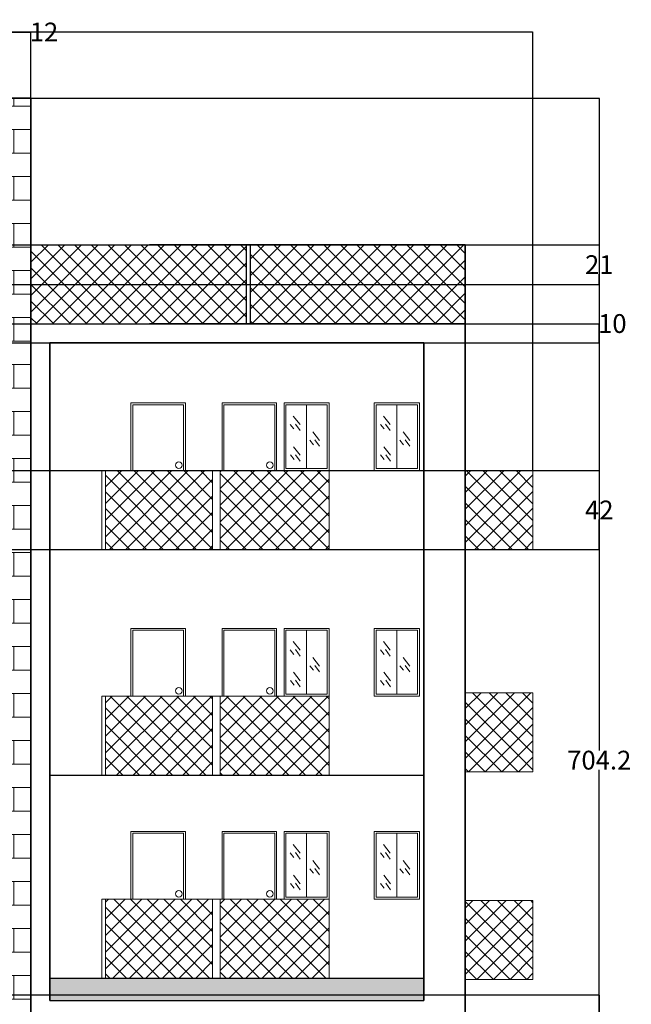
# Model space of a CAD drawing. Units: inches. Extents: x 183 to 891, y 196 to 984.
# Tile 3 of 3: x 566 to 891, y 460 to 984. Entities that reach past the tile are written whole.
import ezdxf

# ---------------------------------------------------------------- set-up
doc = ezdxf.new("R2010")
doc.units = ezdxf.units.IN
doc.header["$MEASUREMENT"] = 0
for name, color, linetype, lineweight in [('A-ANNO-DIMS', 2, 'Continuous', 18), ('A-DOOR', 3, 'Continuous', 20), ('A-FLOR', 7, 'Continuous', 30), ('A-FLOR-PATT', 2, 'Continuous', 13), ('A-GLAZ', 4, 'Continuous', 18), ('A-RAIL', 7, 'Continuous', 20), ('A-RAIL-PATT', 8, 'Continuous', 13), ('A-ROOF', 7, 'Continuous', 25), ('A-WALL', 7, 'Continuous', 35), ('A-WALL-PATT', 251, 'Continuous', 13)]:
    doc.layers.add(name, color=color, linetype=linetype, lineweight=lineweight)
doc.styles.get("Standard").update_dxf_attribs({"font": 'arial.ttf'})
doc.dimstyles.get("Standard").update_dxf_attribs({"dimtxt": 10, "dimasz": 0.18, "dimexe": 0.18, "dimexo": 0.0625, "dimgap": 0.09, "dimtad": 0, "dimtih": 1, "dimtoh": 1, "dimdec": 0, "dimzin": 0, "dimdsep": 46, "dimlunit": 3, "dimtxsty": 'Standard', "dimcen": 0.09, "dimadec": 0, "dimazin": 0, "dimtfac": 1, "dimtdec": 0, "dimtofl": 0, "dimtmove": 0, "dimatfit": 3, "dimfxl": 1, "dimtolj": 1, "dimtzin": 0, "dimarcsym": 0})

# ---------------------------------------------------------------- blocks, each defined once
blk = doc.blocks.new('WIN-SASH-PAIR-22X34')
for p, q in [((11, 34), (11, 0)), ((18.11, 27.96), (14.53, 23.4)), ((16.98, 23.73), (14.53, 20.31)), ((19.74, 23.56), (17.79, 21.12)), ((7.74, 19.54), (4.16, 14.99)), ((6.61, 15.31), (4.16, 11.9)), ((9.37, 15.15), (7.42, 12.71)), ((18.01, 11.64), (14.43, 7.09)), ((16.87, 7.41), (14.43, 4)), ((19.64, 7.25), (17.69, 4.81))]:
    blk.add_line(p, q)
blk.add_lwpolyline([(0, 0), (22, 0), (22, 34), (0, 34)], close=True)
blk = doc.blocks.new('DOOR-BALCONY-ELEV-29')
for p, q in [((0, 0), (0, 36)), ((0, 36), (29, 36)), ((1, 35), (28, 35)), ((1, 0), (1, 35)), ((28, 35), (28, 0)), ((29, 36), (29, 0))]:
    blk.add_line(p, q)
blk.add_circle((3.53, 2.84), 1.74)
blk = doc.blocks.new('*D8')
at = {"layer": 'A-ANNO-DIMS', "color": 0, "lineweight": -2, "transparency": 16777216}
for p, q in [((238.6, 742.93), (238.6, 977.12)), ((238.78, 976.94), (527.45, 976.94)), ((838.42, 976.94), (549.75, 976.94)), ((838.6, 743.74), (838.6, 977.12))]:
    blk.add_line(p, q, dxfattribs=at)
at = {"layer": 'A-ANNO-DIMS', "color": 0, "transparency": 16777216}
for points in [[(238.78, 976.97), (238.78, 976.91), (238.6, 976.94)], [(838.42, 976.97), (838.42, 976.91), (838.6, 976.94)]]:
    blk.add_solid(points, dxfattribs=at)
at = {"layer": 'Defpoints', "color": 0, "transparency": 16777216}
for p in [(838.6, 976.94), (238.6, 742.86), (838.6, 743.68)]:
    blk.add_point(p, dxfattribs=at)
at = {"layer": 'A-ANNO-DIMS', "color": 0, "transparency": 16777216, "insert": (538.6, 976.94), "char_height": 10, "attachment_point": 5}
blk.add_mtext('\\A1;600', dxfattribs=at)
blk = doc.blocks.new('*D9')
at = {"layer": 'A-ANNO-DIMS', "color": 0, "lineweight": -2, "transparency": 16777216}
for p, q in [((571.66, 941.68), (874.04, 941.68)), ((873.86, 941.5), (873.86, 594.79)), ((873.86, 237.69), (873.86, 584.4)), ((802.66, 237.51), (874.04, 237.51))]:
    blk.add_line(p, q, dxfattribs=at)
at = {"layer": 'A-ANNO-DIMS', "color": 0, "transparency": 16777216}
for points in [[(873.83, 941.5), (873.89, 941.5), (873.86, 941.68)], [(873.83, 237.69), (873.89, 237.69), (873.86, 237.51)]]:
    blk.add_solid(points, dxfattribs=at)
at = {"layer": 'Defpoints', "color": 0, "transparency": 16777216}
for p in [(571.6, 941.68), (873.86, 941.68), (802.6, 237.51)]:
    blk.add_point(p, dxfattribs=at)
at = {"layer": 'A-ANNO-DIMS', "color": 0, "transparency": 16777216, "insert": (873.86, 589.59), "char_height": 10, "attachment_point": 5}
blk.add_mtext('\\A1;704.2', dxfattribs=at)
blk = doc.blocks.new('*D37')
at = {"layer": 'A-ANNO-DIMS', "color": 0, "lineweight": -2, "transparency": 16777216}
for p, q in [((559.6, 317.74), (559.6, 977.12)), ((559.78, 976.94), (571.42, 976.94)), ((571.6, 237.57), (571.6, 977.12)), ((571.6, 976.94), (571.78, 976.94))]:
    blk.add_line(p, q, dxfattribs=at)
at = {"layer": 'A-ANNO-DIMS', "color": 0, "transparency": 16777216}
for points in [[(559.78, 976.97), (559.78, 976.91), (559.6, 976.94)], [(571.42, 976.97), (571.42, 976.91), (571.6, 976.94)]]:
    blk.add_solid(points, dxfattribs=at)
at = {"layer": 'Defpoints', "color": 0, "transparency": 16777216}
for p in [(571.6, 976.94), (559.6, 317.68), (571.6, 237.51)]:
    blk.add_point(p, dxfattribs=at)
at = {"layer": 'A-ANNO-DIMS', "color": 0, "transparency": 16777216, "insert": (578.51, 976.94), "char_height": 10, "attachment_point": 5}
blk.add_mtext('\\A1;12', dxfattribs=at)
blk = doc.blocks.new('*D39')
at = {"layer": 'A-ANNO-DIMS', "color": 0, "lineweight": -2, "transparency": 16777216}
for p, q in [((559.66, 464.68), (874.04, 464.68)), ((873.86, 464.5), (873.86, 396.29)), ((873.86, 317.86), (873.86, 386.06)), ((559.66, 317.68), (874.04, 317.68))]:
    blk.add_line(p, q, dxfattribs=at)
at = {"layer": 'A-ANNO-DIMS', "color": 0, "transparency": 16777216}
for points in [[(873.83, 464.5), (873.89, 464.5), (873.86, 464.68)], [(873.83, 317.86), (873.89, 317.86), (873.86, 317.68)]]:
    blk.add_solid(points, dxfattribs=at)
at = {"layer": 'Defpoints', "color": 0, "transparency": 16777216}
for p in [(559.6, 464.68), (873.86, 464.68), (559.6, 317.68)]:
    blk.add_point(p, dxfattribs=at)
at = {"layer": 'A-ANNO-DIMS', "color": 0, "transparency": 16777216, "insert": (873.86, 391.18), "char_height": 10, "attachment_point": 5}
blk.add_mtext('\\A1;147', dxfattribs=at)
blk = doc.blocks.new('*D45')
at = {"layer": 'A-ANNO-DIMS', "color": 0, "lineweight": -2, "transparency": 16777216}
for p, q in [((467.66, 743.68), (874.04, 743.68)), ((873.86, 743.5), (873.86, 727.79)), ((873.86, 701.86), (873.86, 717.56)), ((467.66, 701.68), (874.04, 701.68))]:
    blk.add_line(p, q, dxfattribs=at)
at = {"layer": 'A-ANNO-DIMS', "color": 0, "transparency": 16777216}
for points in [[(873.83, 743.5), (873.89, 743.5), (873.86, 743.68)], [(873.83, 701.86), (873.89, 701.86), (873.86, 701.68)]]:
    blk.add_solid(points, dxfattribs=at)
at = {"layer": 'Defpoints', "color": 0, "transparency": 16777216}
for p in [(467.6, 743.68), (873.86, 743.68), (467.6, 701.68)]:
    blk.add_point(p, dxfattribs=at)
at = {"layer": 'A-ANNO-DIMS', "color": 0, "transparency": 16777216, "insert": (873.86, 722.68), "char_height": 10, "attachment_point": 5}
blk.add_mtext('\\A1;42', dxfattribs=at)
blk = doc.blocks.new('*D48')
at = {"layer": 'A-ANNO-DIMS', "color": 0, "lineweight": -2, "transparency": 16777216}
for p, q in [((499.66, 821.68), (874.04, 821.68)), ((873.86, 821.68), (873.86, 821.86)), ((873.86, 821.86), (874.04, 821.86)), ((873.86, 811.86), (873.86, 821.5)), ((489.66, 811.68), (874.04, 811.68))]:
    blk.add_line(p, q, dxfattribs=at)
at = {"layer": 'A-ANNO-DIMS', "color": 0, "transparency": 16777216}
for points in [[(873.83, 821.5), (873.89, 821.5), (873.86, 821.68)], [(873.83, 811.86), (873.89, 811.86), (873.86, 811.68)]]:
    blk.add_solid(points, dxfattribs=at)
at = {"layer": 'Defpoints', "color": 0, "transparency": 16777216}
for p in [(499.6, 821.68), (873.86, 821.68), (489.6, 811.68)]:
    blk.add_point(p, dxfattribs=at)
at = {"layer": 'A-ANNO-DIMS', "color": 0, "transparency": 16777216, "insert": (880.81, 821.86), "char_height": 10, "attachment_point": 5}
blk.add_mtext('\\A1;10', dxfattribs=at)
blk = doc.blocks.new('*D49')
at = {"layer": 'A-ANNO-DIMS', "color": 0, "lineweight": -2, "transparency": 16777216}
for p, q in [((499.66, 863.68), (874.04, 863.68)), ((873.86, 863.5), (873.86, 858.29)), ((873.86, 842.86), (873.86, 848.06)), ((499.66, 842.68), (874.04, 842.68))]:
    blk.add_line(p, q, dxfattribs=at)
at = {"layer": 'A-ANNO-DIMS', "color": 0, "transparency": 16777216}
for points in [[(873.83, 863.5), (873.89, 863.5), (873.86, 863.68)], [(873.83, 842.86), (873.89, 842.86), (873.86, 842.68)]]:
    blk.add_solid(points, dxfattribs=at)
at = {"layer": 'Defpoints', "color": 0, "transparency": 16777216}
for p in [(499.6, 863.68), (873.86, 863.68), (499.6, 842.68)]:
    blk.add_point(p, dxfattribs=at)
at = {"layer": 'A-ANNO-DIMS', "color": 0, "transparency": 16777216, "insert": (873.86, 853.18), "char_height": 10, "attachment_point": 5}
blk.add_mtext('\\A1;21', dxfattribs=at)

msp = doc.modelspace()

# ---------------------------------------------------------------- hatches: boundary and pattern name
at = {"layer": 'A-FLOR-PATT'}
h = msp.add_hatch(color=256, dxfattribs=at)
h.dxf.hatch_style = 1
h.paths.add_polyline_path([(489.599, 473.6754), (296.599, 473.6754), (296.599, 461.6754), (489.599, 461.6754)])
h.paths.add_polyline_path([(780.599, 473.6754), (581.599, 473.6754), (581.599, 461.6754), (780.599, 461.6754)])
at = {"layer": 'A-RAIL-PATT'}
h = msp.add_hatch(dxfattribs=at)
h.set_pattern_fill('ANSI37', color=256, scale=50)
h.paths.add_polyline_path([(386.099, 842.6754), (274.599, 842.6754), (274.599, 821.6754), (386.099, 821.6754)])
h.paths.add_polyline_path([(386.099, 863.6754), (274.599, 863.6754), (274.599, 842.6754), (386.099, 842.6754)])
h.paths.add_polyline_path([(499.599, 863.6754), (388.099, 863.6754), (388.099, 842.6754), (499.599, 842.6754)])
h.paths.add_polyline_path([(499.599, 842.6754), (388.099, 842.6754), (388.099, 821.6754), (499.599, 821.6754)])
h.paths.add_polyline_path([(686.099, 863.6754), (571.599, 863.6754), (571.599, 842.6754), (686.099, 842.6754)])
h.paths.add_polyline_path([(686.099, 842.6754), (571.599, 842.6754), (571.599, 821.6754), (634.599, 821.6754), (686.099, 821.6754)])
h.paths.add_polyline_path([(802.599, 863.6754), (688.099, 863.6754), (688.099, 842.6754), (802.599, 842.6754)])
h.paths.add_polyline_path([(802.599, 842.6754), (688.099, 842.6754), (688.099, 821.6754), (802.599, 821.6754)])
h = msp.add_hatch(dxfattribs=at)
h.set_pattern_fill('ANSI37', color=256, scale=50)
h.paths.add_polyline_path([(404.599, 743.6754), (346.599, 743.6754), (346.599, 701.6754), (404.599, 701.6754)])
h.paths.add_polyline_path([(465.599, 743.6754), (408.599, 743.6754), (408.599, 701.6754), (465.599, 701.6754)])
h.paths.add_polyline_path([(668.2227, 743.6754), (611.2227, 743.6754), (611.2227, 701.6754), (668.2227, 701.6754)])
h.paths.add_polyline_path([(730.2227, 743.6754), (706.2227, 743.6754), (672.2227, 743.6754), (672.2227, 701.6754), (730.2227, 701.6754)])
h.paths.add_polyline_path([(838.599, 743.6754), (802.599, 743.6754), (802.599, 701.6754), (838.599, 701.6754)])
h.paths.add_polyline_path([(274.599, 742.8641), (238.599, 742.8641), (238.599, 700.8641), (274.599, 700.8641)])
h.paths.add_polyline_path([(274.599, 625.2404), (238.599, 625.2404), (238.599, 583.2404), (274.599, 583.2404)])
h.paths.add_polyline_path([(404.599, 623.6754), (346.599, 623.6754), (346.599, 581.6754), (404.599, 581.6754)])
h.paths.add_polyline_path([(465.599, 623.6754), (408.599, 623.6754), (408.599, 581.6754), (465.599, 581.6754)])
h.paths.add_polyline_path([(668.2227, 623.6754), (611.2227, 623.6754), (611.2227, 581.6754), (668.2227, 581.6754)])
h.paths.add_polyline_path([(730.2227, 623.6754), (672.2227, 623.6754), (672.2227, 581.6754), (730.2227, 581.6754)])
h.paths.add_polyline_path([(838.599, 625.42), (802.599, 625.42), (802.599, 583.42), (838.599, 583.42)])
h.paths.add_polyline_path([(404.599, 515.6754), (346.599, 515.6754), (346.599, 473.6754), (404.599, 473.6754)])
h.paths.add_polyline_path([(465.599, 515.6754), (408.599, 515.6754), (408.599, 473.6754), (465.599, 473.6754)])
h.paths.add_polyline_path([(668.2227, 515.6754), (611.2227, 515.6754), (611.2227, 473.6754), (668.2227, 473.6754)])
h.paths.add_polyline_path([(730.2227, 515.6754), (706.2227, 515.6754), (672.2227, 515.6754), (672.2227, 473.6754), (730.2227, 473.6754)])
h.paths.add_polyline_path([(838.599, 514.8979), (802.599, 514.8979), (802.599, 472.8979), (838.599, 472.8979)])
h.paths.add_polyline_path([(668.2227, 383.6754), (611.2227, 383.6754), (611.2227, 341.6754), (668.2227, 341.6754)])
h.paths.add_polyline_path([(609.2227, 383.6754), (571.599, 383.6754), (571.599, 341.6754), (601.2227, 341.6754), (609.2227, 341.6754)])
h.paths.add_polyline_path([(730.2227, 383.6754), (672.2227, 383.6754), (672.2227, 341.6754), (730.2227, 341.6754)])
h.paths.add_polyline_path([(838.599, 383.6754), (802.599, 383.6754), (802.599, 341.6754), (838.599, 341.6754)])
h.paths.add_polyline_path([(499.599, 383.6754), (467.599, 383.6754), (467.599, 341.6754), (499.599, 341.6754)])
h.paths.add_polyline_path([(465.599, 383.6754), (408.599, 383.6754), (408.599, 341.6754), (465.599, 341.6754)])
h.paths.add_polyline_path([(404.599, 383.6754), (346.599, 383.6754), (346.599, 341.6754), (404.599, 341.6754)])
h.paths.add_polyline_path([(274.599, 383.6754), (238.599, 383.6754), (238.599, 341.6754), (274.599, 341.6754)])
h.paths.add_polyline_path([(274.599, 514.3451), (238.599, 514.3451), (238.599, 472.3451), (274.599, 472.3451)])
at = {"layer": 'A-WALL-PATT'}
h = msp.add_hatch(dxfattribs=at)
h.set_pattern_fill('BRICK', color=256, scale=50)
h.paths.add_polyline_path([(571.599, 341.6754), (571.599, 821.6754), (571.599, 905.6754), (571.599, 941.6754), (499.599, 941.6754), (499.599, 905.6754), (499.599, 821.6754), (499.599, 341.6754), (499.599, 237.5076), (571.599, 237.5076)])
h.paths.add_polyline_path([(511.599, 317.6754), (511.599, 905.6754), (559.599, 905.6754), (559.599, 317.6754)], flags=16)

# ---------------------------------------------------------------- linework, layer by layer
at = {"layer": 'A-FLOR'}
for p, q in [((581.599, 701.6754), (780.599, 701.6754)), ((581.599, 581.6754), (780.599, 581.6754)), ((581.599, 473.6754), (780.599, 473.6754)), ((581.599, 461.6754), (780.599, 461.6754))]:
    msp.add_line(p, q, dxfattribs=at)
at = {"layer": 'A-GLAZ'}
for p, q in [((763.2227, 743.6754), (754.2227, 743.6754)), ((763.2227, 623.6754), (754.2227, 623.6754)), ((763.2227, 515.6754), (754.2227, 515.6754))]:
    msp.add_line(p, q, dxfattribs=at)
for points in [[(730.2227, 743.6754), (706.2227, 743.6754), (706.2227, 779.6754), (730.2227, 779.6754)], [(778.2227, 743.6754), (754.2227, 743.6754), (754.2227, 779.6754), (778.2227, 779.6754)], [(730.2227, 623.6754), (706.2227, 623.6754), (706.2227, 659.6754), (730.2227, 659.6754)], [(778.2227, 623.6754), (754.2227, 623.6754), (754.2227, 659.6754), (778.2227, 659.6754)], [(730.2227, 515.6754), (706.2227, 515.6754), (706.2227, 551.6754), (730.2227, 551.6754)], [(778.2227, 515.6754), (754.2227, 515.6754), (754.2227, 551.6754), (778.2227, 551.6754)]]:
    msp.add_lwpolyline(points, close=True, dxfattribs=at)
at = {"layer": 'A-RAIL'}
for p, q in [((730.2227, 743.6754), (609.2227, 743.6754)), ((609.2227, 701.6754), (609.2227, 743.6754)), ((609.2227, 743.6754), (730.2227, 743.6754)), ((611.2227, 701.6754), (611.2227, 743.6754)), ((668.2227, 743.4954), (668.2227, 701.6754)), ((672.2227, 743.4954), (672.2227, 701.6754)), ((730.2227, 743.6754), (730.2227, 701.6754)), ((838.599, 743.6754), (802.599, 743.6754)), ((838.599, 701.6754), (838.599, 743.6754)), ((802.599, 701.6754), (838.599, 701.6754)), ((609.2227, 623.6754), (730.2227, 623.6754)), ((730.2227, 623.6754), (609.2227, 623.6754)), ((609.2227, 581.6754), (609.2227, 623.6754)), ((611.2227, 581.6754), (611.2227, 623.6754)), ((668.2227, 623.4954), (668.2227, 581.6754)), ((672.2227, 623.4954), (672.2227, 581.6754)), ((730.2227, 623.6754), (730.2227, 581.6754)), ((838.599, 625.42), (802.599, 625.42)), ((838.599, 583.42), (838.599, 625.42)), ((802.599, 583.42), (838.599, 583.42)), ((730.2227, 515.6754), (609.2227, 515.6754)), ((609.2227, 473.6754), (609.2227, 515.6754)), ((611.2227, 473.6754), (611.2227, 515.6754)), ((668.2227, 515.4954), (668.2227, 473.6754)), ((672.2227, 515.4954), (672.2227, 473.6754)), ((730.2227, 515.6754), (730.2227, 473.6754)), ((838.599, 514.8979), (802.599, 514.8979)), ((838.599, 472.8979), (838.599, 514.8979)), ((802.599, 472.8979), (838.599, 472.8979))]:
    msp.add_line(p, q, dxfattribs=at)
at = {"layer": 'A-ROOF'}
for p, q in [((571.599, 863.6754), (634.599, 863.6754)), ((571.599, 863.6754), (802.599, 863.6754)), ((802.599, 863.6754), (634.599, 863.6754)), ((686.099, 863.6754), (686.099, 821.6754)), ((688.099, 863.6754), (688.099, 821.6754)), ((571.599, 842.6754), (802.599, 842.6754)), ((571.599, 821.6754), (634.599, 821.6754)), ((802.599, 821.6754), (634.599, 821.6754))]:
    msp.add_line(p, q, dxfattribs=at)
at = {"layer": 'A-WALL'}
for p, q in [((499.599, 941.6754), (571.599, 941.6754)), ((571.599, 941.6754), (571.599, 905.6754)), ((571.599, 905.6754), (571.599, 821.6754)), ((802.599, 237.5076), (802.599, 863.6754)), ((571.599, 821.6754), (571.599, 341.6754)), ((581.599, 811.6754), (581.599, 461.6754)), ((780.599, 811.6754), (581.599, 811.6754)), ((780.599, 461.6754), (780.599, 811.6754))]:
    msp.add_line(p, q, dxfattribs=at)

# ---------------------------------------------------------------- block references
at = {"layer": 'A-DOOR', "extrusion": (0, 0, -1), "zscale": -1}
for p in [(-653.7962, 743.675), (-702.2227, 743.675), (-653.7962, 623.675), (-702.2227, 623.675), (-653.7962, 515.675), (-702.2227, 515.675)]:
    msp.add_blockref('DOOR-BALCONY-ELEV-29', p, dxfattribs=at)
at = {"layer": 'A-GLAZ', "extrusion": (0, 0, -1), "zscale": -1}
for p in [(-729.2227, 744.675), (-777.2227, 744.675), (-729.2227, 624.675), (-777.2227, 624.675), (-729.2227, 516.675), (-777.2227, 516.675)]:
    msp.add_blockref('WIN-SASH-PAIR-22X34', p, dxfattribs=at)

# ---------------------------------------------------------------- dimensions: what is measured, and where the dimension line sits
at = {"layer": 'A-ANNO-DIMS'}
for base, p1, p2, picture, middle in [((838.599, 976.9404), (238.599, 742.8641), (838.599, 743.6754), '*D8', (538.599, 976.9404)), ((571.599, 976.9404), (559.599, 317.6754), (571.599, 237.5076), '*D37', (578.5095, 976.9404))]:
    dim = msp.add_linear_dim(base=base, p1=p1, p2=p2, dimstyle='Standard', override={"dimdec": 0, "dimlfac": 1, "dimrnd": 0, "dimzin": 0, "dimdsep": 46, "dimlunit": 2}, dxfattribs=at)
    dim.commit()
    dim.dimension.update_dxf_attribs({"geometry": picture, "text_midpoint": middle})
for base, p1, p2, override, picture, middle in [((873.864, 941.6754), (802.599, 237.5076), (571.599, 941.6754), {"dimdec": 1, "dimlfac": 1, "dimrnd": 0, "dimzin": 0, "dimdsep": 46, "dimlunit": 2}, '*D9', (873.864, 589.5915)), ((873.864, 863.6754), (499.599, 842.6754), (499.599, 863.6754), {"dimdec": 0, "dimlfac": 1, "dimrnd": 0, "dimzin": 0, "dimdsep": 46, "dimlunit": 2}, '*D49', (873.864, 853.1754)), ((873.864, 821.6754), (489.599, 811.6754), (499.599, 821.6754), {"dimdec": 0, "dimlfac": 1, "dimrnd": 0, "dimzin": 0, "dimdsep": 46, "dimlunit": 2}, '*D48', (880.8086, 821.8554)), ((873.864, 743.6754), (467.599, 701.6754), (467.599, 743.6754), {"dimdec": 0, "dimlfac": 1, "dimrnd": 0, "dimzin": 0, "dimdsep": 46, "dimlunit": 2}, '*D45', (873.864, 722.6754)), ((873.864, 464.6754), (559.599, 317.6754), (559.599, 464.6754), {"dimdec": 0, "dimlfac": 1, "dimrnd": 0, "dimzin": 0, "dimdsep": 46, "dimlunit": 2}, '*D39', (873.864, 391.1754))]:
    dim = msp.add_linear_dim(base=base, p1=p1, p2=p2, angle=90, dimstyle='Standard', override=override, dxfattribs=at)
    dim.commit()
    dim.dimension.update_dxf_attribs({"geometry": picture, "text_midpoint": middle})

doc.saveas('drawing.dxf')
